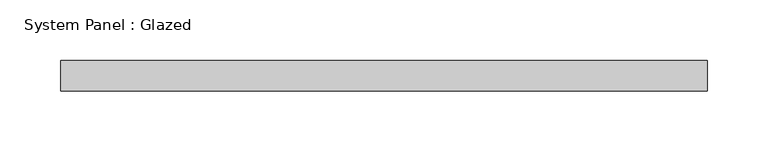
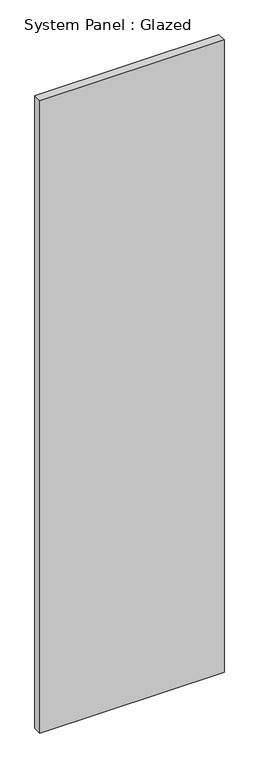
"""IFC4 building model written with IfcOpenShell, lengths in millimetres: plate geometry, System Panel : Glazed."""

from ifc_helpers import new_model, si_unit, origin, origin_with_axes, place, context, project, spatial, polyline, outline, extrude, source, transform, mapped, element, save


def system_panel_glazed_d76279c0(model_context):
    return source(origin(), model_context, "Body", "SweptSolid", [
        extrude(outline(polyline([(266.7, 19.05), (-266.7, 19.05), (-266.7, 44.45), (266.7, 44.45), (266.7, 19.05)])), origin_with_axes(), (0.0, 0.0, 1.0), 1936.6147749),
    ])


if __name__ == "__main__":
    model = new_model("IFC4")
    model_context = context("Model", 3, world=origin())
    ifc_project = project(units=[si_unit("LENGTHUNIT", "METRE", prefix="MILLI")], contexts=[model_context])
    site = spatial("IfcSite", under=ifc_project)
    building = spatial("IfcBuilding", under=site)
    placement = place(None, origin())
    system_panel_glazed_shape = system_panel_glazed_d76279c0(model_context)
    element("IfcPlate", 1, ObjectType="System Panel : Glazed", at=placement, inside=building, context=model_context, shape_type="MappedRepresentation", body=[
        mapped(system_panel_glazed_shape, transform((0.0, 0.0, 0.0), x_axis=(1.0, 0.0, 0.0), y_axis=(0.0, 1.0, 0.0), z_axis=(0.0, 0.0, 1.0))),
    ])
    save(model, "model.ifc")

# Revit data of these elements
# Type "System Panel : Glazed"
#   Construction Type Id = "GSP4R"
#   Analytic Construction = "1/8 in Pilkington single glazing"
#   Visual Light Transmittance = 0.9
#   Solar Heat Gain Coefficient = 0.86
#   Heat Transfer Coefficient (U) = 1.18115 BTU/(h·ft²·°F)
#   Define Thermal Properties by = 1
# Element 1 (IfcPlate, "System Panel : Glazed")
#   Materials on its faces: "Glass"
# Materials
#   "Glass": class "Glass", colour RGB 0 128 192, transparency 0.75, Description = "Soda Lime Glass", Cost = 0
